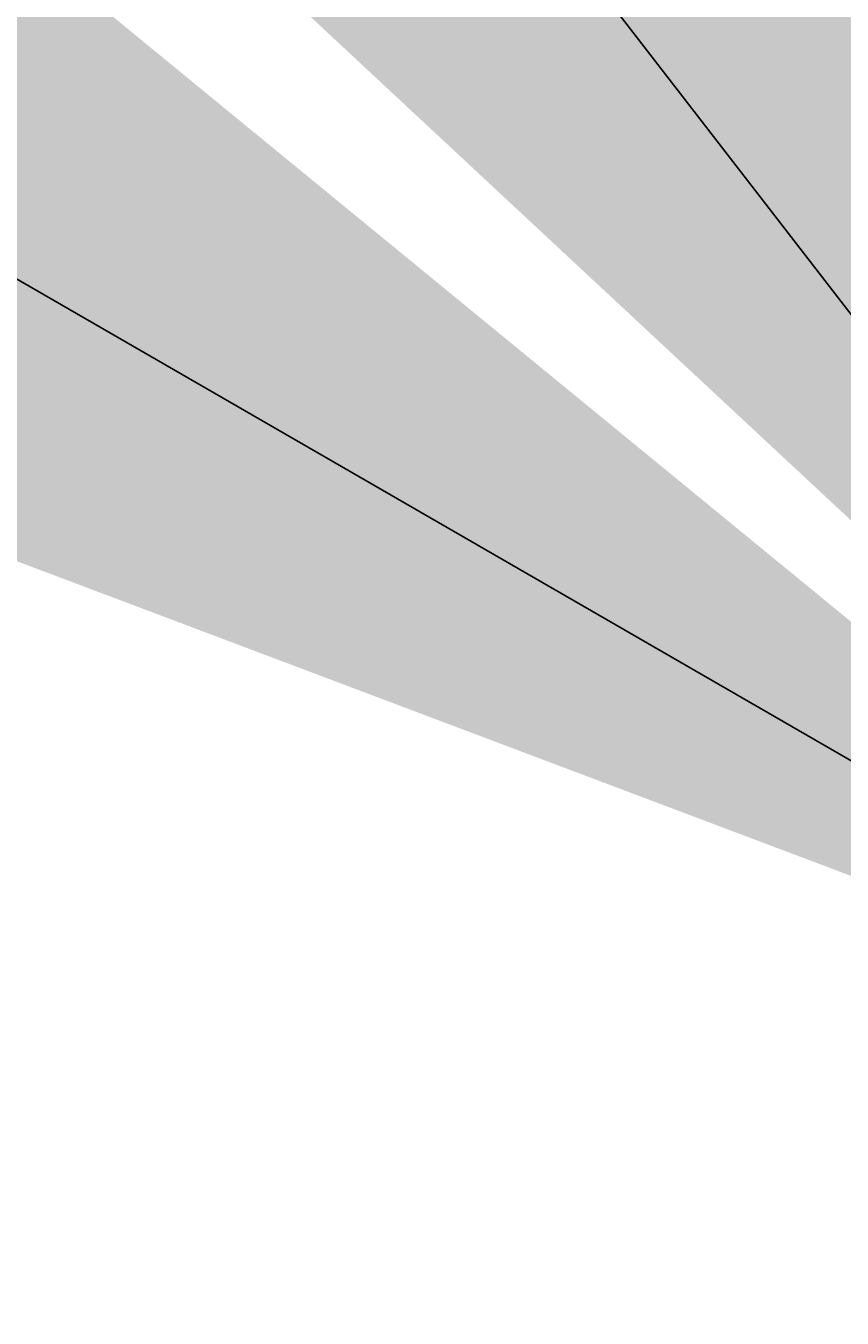
# Model space of a CAD drawing. Units: inches. Extents: x -9413 to 9703, y -9719 to 9096.
# Tile 1 of 1: x -2479 to -993, y -311 to 2041. Entities that reach past the tile are written whole.
import ezdxf
from ezdxf import colors
from ezdxf.entities.mleader import LeaderData, LeaderLine
from ezdxf.math import Vec2, Vec3

# ---------------------------------------------------------------- set-up
doc = ezdxf.new("R2010")
doc.units = ezdxf.units.IN
doc.header["$MEASUREMENT"] = 0
doc.layers.add('M-ANNO-TEXT', color=7, linetype='Continuous', lineweight=18)
doc.styles.get("Standard").update_dxf_attribs({"font": 'arial.ttf'})

msp = doc.modelspace()

# ---------------------------------------------------------------- leaders
at = {"layer": 'M-ANNO-TEXT'}
ml = msp.add_multileader_mtext('Standard', dxfattribs=at)
ml.set_content('steam drum', color=256)
ml.set_leader_properties()
ml.build(insert=Vec2(0, 0))
ml.multileader.update_dxf_attribs({"dogleg_length": 0.36, "arrow_head_size": 10000, "scale": 10})
ctx = ml.context
ctx.base_point, ctx.scale, ctx.char_height, ctx.arrow_head_size, ctx.landing_gap_size, ctx.plane_origin = Vec3(1.078100315116472, 187.1657656808087), 10, 5.4, 10000, 0.9, Vec3(56.53630785249729, 178.1917761520126)
ctx.text_align_type = 2
notes = []
notes.append((ctx, [(0, (1, 1, 0), (49.60206616053652, 187.1657656808087), (-1, 0), 7.616326009130828, [(0, [(56.5363078524973, 178.1917761520126)], 0, [])])]))
ctx.mtext.insert, ctx.mtext.alignment, ctx.mtext.flow_direction = Vec3(41.08574015140569, 189.9099675907678), 3, 5
ml = msp.add_multileader_mtext('Standard', dxfattribs=at)
ml.set_content('Boiler', color=256)
ml.set_leader_properties()
ml.build(insert=Vec2(0, 0))
ml.multileader.update_dxf_attribs({"dogleg_length": 0.36, "arrow_head_size": 10000, "scale": 10})
ctx = ml.context
ctx.base_point, ctx.scale, ctx.char_height, ctx.arrow_head_size, ctx.landing_gap_size, ctx.plane_origin = Vec3(31.04430257849453, 103.0991380116177), 10, 5.4, 10000, 0.9, Vec3(69.11352005531556, 99.3051261342938)
ctx.text_align_type = 2
notes.append((ctx, [(0, (1, 1, 0), (62.54209871927075, 103.0991380116177), (-1, 0), 10.86041551321825, [(0, [(69.11352005531556, 99.3051261342938)], 0, [])])]))
ctx.mtext.insert, ctx.mtext.alignment, ctx.mtext.flow_direction = Vec3(50.7816832060525, 105.8433399215768), 3, 5
ml = msp.add_multileader_mtext('Standard', dxfattribs=at)
ml.set_content('Air preheater', color=256)
ml.set_leader_properties()
ml.build(insert=Vec2(0, 0))
ml.multileader.update_dxf_attribs({"dogleg_length": 0.36, "arrow_head_size": 10000, "scale": 10})
ctx = ml.context
ctx.base_point, ctx.scale, ctx.char_height, ctx.arrow_head_size, ctx.landing_gap_size, ctx.plane_origin = Vec3(229.7079293124727, 37.30650895205824), 10, 5.4, 10000, 0.9, Vec3(241.9833706008503, 78.04556948044049)
notes.append((ctx, [(1, (1, 1, 0), (223.7048975654645, 37.30650895205824), (1, 0), 6.003031747008185, [(0, [(241.9833706008503, 78.04556948044049)], 0, [])])]))
ctx.mtext.insert, ctx.mtext.flow_direction = Vec3(230.6079293124727, 40.75609967511417), 5
for ctx, leaders in notes:
    for number, flags, end, landing, length, lines in leaders:
        leader = LeaderData()
        leader.index, (leader.has_last_leader_line, leader.has_dogleg_vector, leader.attachment_direction) = number, flags
        leader.last_leader_point, leader.dogleg_vector, leader.dogleg_length = Vec3(end), Vec3(landing), length
        for number, points, colour, breaks in lines:
            line = LeaderLine()
            line.index, line.vertices, line.color, line.breaks = number, Vec3.list(points), colors.encode_raw_color(colour), breaks
            leader.lines.append(line)
        ctx.leaders.append(leader)

doc.saveas('drawing.dxf')
